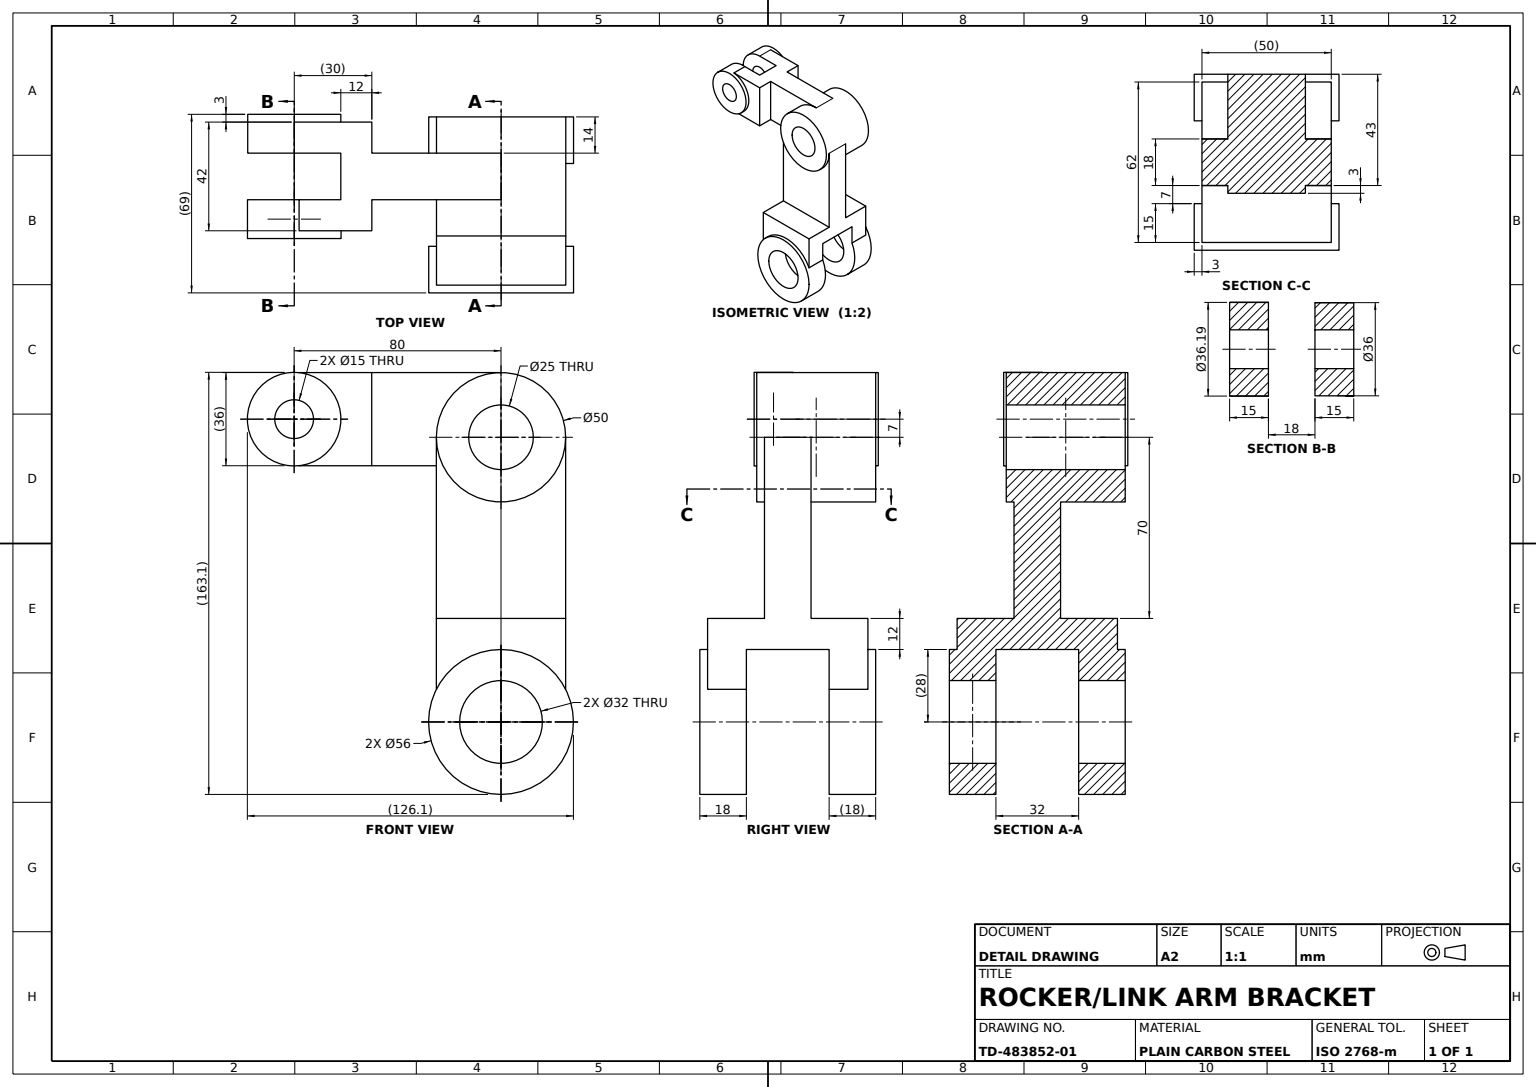
from build123d import *

# Parameters (mm, degrees)
BASE_PLATE_SKETCH_W              = 62
BASE_PLATE_SKETCH_H              = 50
BASE_PLATE_62X50X12_DEPTH        = 12
COLUMN_SKETCH_W                  = 18
COLUMN_SKETCH_H                  = 50
COLUMN_9X9_DEPTH                 = 70
UPPER_HUB_DEPTH                  = 3
UPPER_HUB_DEPTH_BACK             = 43
UPPER_HUB_SKETCH_R               = 25
UPPER_HUB_SKETCH_R_2             = 12.5
LOWER_EAR_A_BLOCK_SKETCH_W       = 50
LOWER_EAR_A_BLOCK_SKETCH_H       = 28
LOWER_EAR_A_BLOCK_DEPTH          = 15
LOWER_EAR_A_ROUND_END_DEPTH      = 3
LOWER_EAR_A_ROUND_END_DEPTH_BACK = 15
LOWER_EAR_A_ROUND_END_SKETCH_R   = 28
LOWER_EAR_A_ROUND_END_SKETCH_R_2 = 16
LOWER_EAR_A_PIN_HOLE_SKETCH_R    = 16
LOWER_EAR_A_PIN_HOLE_DEPTH       = 15
LOWER_EAR_B_BLOCK_SKETCH_W       = 50
LOWER_EAR_B_BLOCK_SKETCH_H       = 28
LOWER_EAR_B_BLOCK_DEPTH          = 15
LOWER_EAR_B_ROUND_END_DEPTH      = 3
LOWER_EAR_B_ROUND_END_DEPTH_BACK = 15
LOWER_EAR_B_ROUND_END_SKETCH_R   = 28
LOWER_EAR_B_ROUND_END_SKETCH_R_2 = 16
LOWER_START                      = -15
LOWER_EAR_B_PIN_HOLE_SKETCH_R    = 16
LOWER_EAR_B_PIN_HOLE_DEPTH       = 15
UPPER_BRACKET_BLOCK_DEPTH        = 25
UPPER_BRACKET_BLOCK_DEPTH_BACK   = 25
UPPER_BRACKET_BLOCK_SKETCH_W     = 18
UPPER_BRACKET_BLOCK_SKETCH_H     = 36
UPPER_CLEVIS_ARM_SKETCH_W        = 42
UPPER_CLEVIS_ARM_SKETCH_H        = 36
UPPER_CLEVIS_ARM_DEPTH           = 30
CLEVIS_SLOT_SKETCH_W             = 18
CLEVIS_SLOT_SKETCH_H             = 36
CLEVIS_SLOT_12X12_DEPTH          = 18
UPPER_EAR_A_ROUND_END_DEPTH      = 3
UPPER_EAR_A_ROUND_END_DEPTH_BACK = 12
UPPER_EAR_A_ROUND_END_SKETCH_R   = 18.096202238
UPPER_EAR_A_ROUND_END_SKETCH_R_2 = 7.5
UPPER_EAR_A_PIN_HOLE_SKETCH_R    = 7.5
UPPER_EAR_A_PIN_HOLE_DEPTH       = 12
UPPER_EAR_B_ROUND_END_DEPTH      = 3
UPPER_EAR_B_ROUND_END_DEPTH_BACK = 12
UPPER_EAR_B_ROUND_END_SKETCH_R   = 18
UPPER_EAR_B_ROUND_END_SKETCH_R_2 = 7.5
UPPER_START                      = -12
UPPER_EAR_B_PIN_HOLE_SKETCH_R    = 7.5
UPPER_EAR_B_PIN_HOLE_DEPTH       = 12
HUB_BORE_SKETCH_R                = 12.5
HUB_BORE_THROUGH_DEPTH           = 66


with BuildPart() as part:
    # Base Plate Sketch → Base Plate 62x50x12 (new body)
    with BuildSketch(Plane(origin=(0, 0, 0), x_dir=(1, 0, 0), z_dir=(0, 1, 0))):
        Rectangle(BASE_PLATE_SKETCH_W, BASE_PLATE_SKETCH_H)
    extrude(amount=BASE_PLATE_62X50X12_DEPTH)

    # Column Sketch → Column 9x9 (add)
    with BuildSketch(Plane(origin=(0, 12, 0), x_dir=(1, 0, 0), z_dir=(0, 1, 0))):
        Rectangle(COLUMN_SKETCH_W, COLUMN_SKETCH_H)
    extrude(amount=COLUMN_9X9_DEPTH)

    # Upper Hub Sketch → Upper Hub (add, two sides: drawn at the far end of the back side and taken through both)
    with BuildSketch(Plane(origin=(9, 0, 0), x_dir=(0, 0, -1), z_dir=(1, 0, 0)).offset(-UPPER_HUB_DEPTH_BACK)):
        with Locations((0, 82)):
            Circle(UPPER_HUB_SKETCH_R)
        with Locations((0, 82)):
            Circle(UPPER_HUB_SKETCH_R_2, mode=Mode.SUBTRACT)
    extrude(amount=UPPER_HUB_DEPTH + UPPER_HUB_DEPTH_BACK)

    # Lower Ear A Block Sketch → Lower Ear A Block (add)
    with BuildSketch(Plane(origin=(31, 0, 0), x_dir=(0, 0, -1), z_dir=(1, 0, 0))):
        with Locations((0, -14)):
            Rectangle(LOWER_EAR_A_BLOCK_SKETCH_W, LOWER_EAR_A_BLOCK_SKETCH_H)
    extrude(amount=-LOWER_EAR_A_BLOCK_DEPTH)

    # Lower Ear A Round End Sketch → Lower Ear A Round End (add, two sides: drawn at the far end of the back side and taken through both)
    with BuildSketch(Plane(origin=(31, 0, 0), x_dir=(0, 0, -1), z_dir=(1, 0, 0)).offset(-LOWER_EAR_A_ROUND_END_DEPTH_BACK)):
        with Locations(Location((0, -28, 0), (0, 0, 153.234499423))):
            Circle(LOWER_EAR_A_ROUND_END_SKETCH_R)
        with Locations((0, -28)):
            Circle(LOWER_EAR_A_ROUND_END_SKETCH_R_2, mode=Mode.SUBTRACT)
    extrude(amount=LOWER_EAR_A_ROUND_END_DEPTH + LOWER_EAR_A_ROUND_END_DEPTH_BACK)

    # Lower Ear A Pin Hole Sketch → Lower Ear A Pin Hole (cut)
    with BuildSketch(Plane(origin=(31, 0, 0), x_dir=(0, 0, -1), z_dir=(1, 0, 0))):
        with Locations((0, -28)):
            Circle(LOWER_EAR_A_PIN_HOLE_SKETCH_R)
    extrude(amount=-LOWER_EAR_A_PIN_HOLE_DEPTH, mode=Mode.SUBTRACT)

    # Lower Ear B Block Sketch → Lower Ear B Block (add)
    with BuildSketch(Plane.ZY.offset(31)):
        with Locations((0, -14)):
            Rectangle(LOWER_EAR_B_BLOCK_SKETCH_W, LOWER_EAR_B_BLOCK_SKETCH_H)
    extrude(amount=-LOWER_EAR_B_BLOCK_DEPTH)

    # Lower Ear B Round End Sketch → Lower Ear B Round End (add, two sides: drawn at the far end of the back side and taken through both)
    with BuildSketch(Plane.ZY.offset(31).offset(-LOWER_EAR_B_ROUND_END_DEPTH_BACK)):
        with Locations(Location((0, -28, 0), (0, 0, 26.765500577))):
            Circle(LOWER_EAR_B_ROUND_END_SKETCH_R)
        with Locations(Location((0, -28, 0), (0, 0, 180))):
            Circle(LOWER_EAR_B_ROUND_END_SKETCH_R_2, mode=Mode.SUBTRACT)
    extrude(amount=LOWER_EAR_B_ROUND_END_DEPTH + LOWER_EAR_B_ROUND_END_DEPTH_BACK)

    # Lower Ear B Pin Hole Sketch → Lower Ear B Pin Hole (cut)
    with BuildSketch(Plane.ZY.offset(31).offset(LOWER_START)):
        with Locations(Location((0, -28, 0), (0, 0, 180))):
            Circle(LOWER_EAR_B_PIN_HOLE_SKETCH_R)
    extrude(amount=LOWER_EAR_B_PIN_HOLE_DEPTH, mode=Mode.SUBTRACT)

    # Upper Bracket Block Sketch → Upper Bracket Block (add, two sides: drawn at the far end of the back side and taken through both)
    with BuildSketch(Plane.XY.offset(25).offset(-UPPER_BRACKET_BLOCK_DEPTH_BACK)):
        with Locations((-11, 89)):
            Rectangle(UPPER_BRACKET_BLOCK_SKETCH_W, UPPER_BRACKET_BLOCK_SKETCH_H)
    extrude(amount=UPPER_BRACKET_BLOCK_DEPTH + UPPER_BRACKET_BLOCK_DEPTH_BACK)

    # Upper Clevis Arm Sketch → Upper Clevis Arm (add)
    with BuildSketch(Plane.XY.offset(50)):
        with Locations((-11, 89)):
            Rectangle(UPPER_CLEVIS_ARM_SKETCH_W, UPPER_CLEVIS_ARM_SKETCH_H)
    extrude(amount=UPPER_CLEVIS_ARM_DEPTH)

    # Clevis Slot Sketch → Clevis Slot 12x12 (cut)
    with BuildSketch(Plane.XY.offset(80)):
        with Locations((-11, 89)):
            Rectangle(CLEVIS_SLOT_SKETCH_W, CLEVIS_SLOT_SKETCH_H)
    extrude(amount=-CLEVIS_SLOT_12X12_DEPTH, mode=Mode.SUBTRACT)

    # Upper Ear A Round End Sketch → Upper Ear A Round End (add, two sides: drawn at the far end of the back side and taken through both)
    with BuildSketch(Plane(origin=(10, 0, 0), x_dir=(0, 0, -1), z_dir=(1, 0, 0)).offset(-UPPER_EAR_A_ROUND_END_DEPTH_BACK)):
        with Locations(Location((-80, 89, 0), (0, 0, 275.910566162))):
            Circle(UPPER_EAR_A_ROUND_END_SKETCH_R)
        with Locations(Location((-80, 89, 0), (0, 0, 90))):
            Circle(UPPER_EAR_A_ROUND_END_SKETCH_R_2, mode=Mode.SUBTRACT)
    extrude(amount=UPPER_EAR_A_ROUND_END_DEPTH + UPPER_EAR_A_ROUND_END_DEPTH_BACK)

    # Upper Ear A Pin Hole Sketch → Upper Ear A Pin Hole (cut)
    with BuildSketch(Plane(origin=(10, 0, 0), x_dir=(0, 0, -1), z_dir=(1, 0, 0))):
        with Locations(Location((-80, 89, 0), (0, 0, 90))):
            Circle(UPPER_EAR_A_PIN_HOLE_SKETCH_R)
    extrude(amount=-UPPER_EAR_A_PIN_HOLE_DEPTH, mode=Mode.SUBTRACT)

    # Upper Ear B Round End Sketch → Upper Ear B Round End (add, two sides: drawn at the far end of the back side and taken through both)
    with BuildSketch(Plane.ZY.offset(32).offset(-UPPER_EAR_B_ROUND_END_DEPTH_BACK)):
        with Locations(Location((80, 89, 0), (0, 0, 270))):
            Circle(UPPER_EAR_B_ROUND_END_SKETCH_R)
        with Locations(Location((80, 89, 0), (0, 0, 90))):
            Circle(UPPER_EAR_B_ROUND_END_SKETCH_R_2, mode=Mode.SUBTRACT)
    extrude(amount=UPPER_EAR_B_ROUND_END_DEPTH + UPPER_EAR_B_ROUND_END_DEPTH_BACK)

    # Upper Ear B Pin Hole Sketch → Upper Ear B Pin Hole (cut)
    with BuildSketch(Plane.ZY.offset(32).offset(UPPER_START)):
        with Locations(Location((80, 89, 0), (0, 0, 90))):
            Circle(UPPER_EAR_B_PIN_HOLE_SKETCH_R)
    extrude(amount=UPPER_EAR_B_PIN_HOLE_DEPTH, mode=Mode.SUBTRACT)

    # Hub Bore Sketch → Hub Bore Through (cut)
    with BuildSketch(Plane.ZY.offset(34)):
        with Locations(Location((0, 82, 0), (0, 0, 180))):
            Circle(HUB_BORE_SKETCH_R)
    extrude(amount=-HUB_BORE_THROUGH_DEPTH, mode=Mode.SUBTRACT)


solid = part.part
